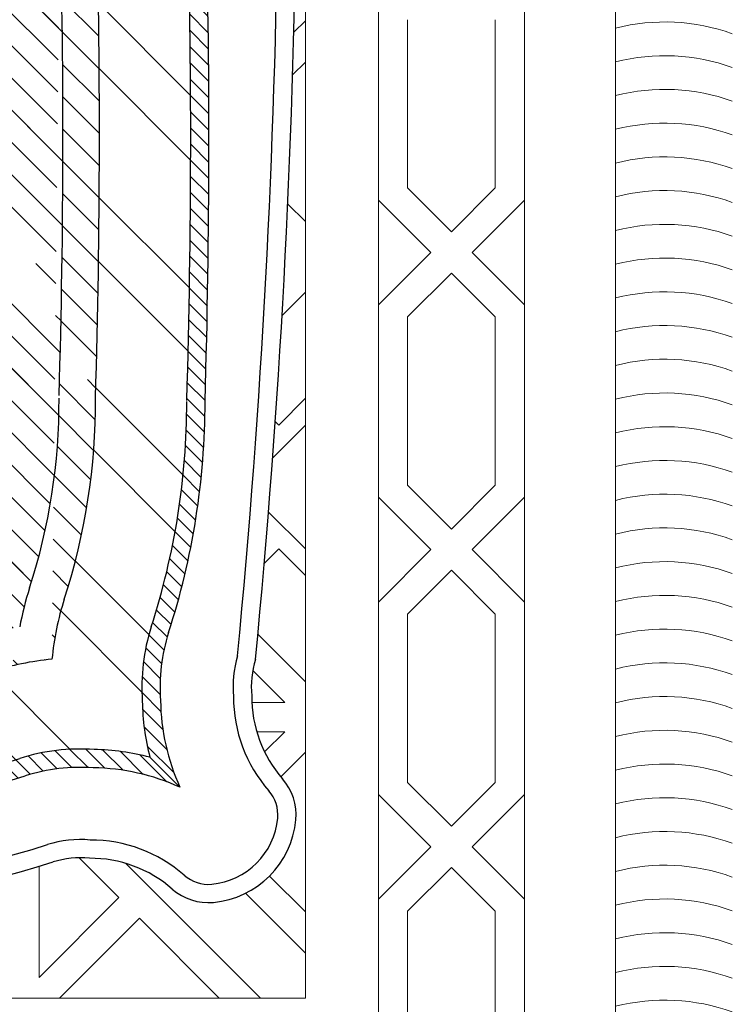
# Model space of a CAD drawing. Units: inches. Extents: x 3592 to 4861, y 1650 to 2243.
# Tile 7 of 30: x 4207.34 to 4219.05, y 1916.11 to 1932.29. Entities that reach past the tile are written whole.
import ezdxf

# ---------------------------------------------------------------- set-up
doc = ezdxf.new("R2010")
doc.units = ezdxf.units.IN
doc.layers.add('A-FURN', color=9, linetype='Continuous', lineweight=13)
doc.layers.add('RA-AP-01$0$INT', color=35, linetype='Continuous', lineweight=5)
for name, color, linetype in [('RA-AP-01$0$FURN', 3, 'Continuous'), ('RA-AP-01$0$WOOD', 64, 'Continuous'), ('RA-AP-02$0$FLPT', 30, 'Continuous')]:
    doc.layers.add(name, color=color, linetype=linetype)

# ---------------------------------------------------------------- blocks, each defined once
blk = doc.blocks.new('A$C67D63ADA')
at = {"layer": 'RA-AP-01$0$INT'}
for p, q in [((5.040068427138238, -6.243416270339336), (5.068754718634292, -6.272102561844619)), ((5.097441010123072, -6.243416270339336), (5.068754718627016, -6.272102561844619)), ((5.202896854247523, -6.243416270324172), (5.231583145752804, -6.272102561820228)), ((5.260269437248857, -6.243416270339973), (5.231583145752802, -6.272102561845255)), ((5.36572528136967, -6.243416270319609), (5.394411572874951, -6.272102561815665)), ((5.394411572874951, -6.272102561815665), (5.423097864372064, -6.243416270309323)), ((5.033441010139864, -6.25941627034044), (4.941240000013775, -6.259416270325027)), ((5.033441010139864, -6.25941627034044), (5.057441010133491, -6.283416270341786)), ((5.104068427125523, -6.259416270336362), (5.080068427127819, -6.283416270341786)), ((5.104068427125523, -6.259416270336362), (5.196269437247836, -6.259416270320948)), ((5.196269437247836, -6.259416270320948), (5.220269437255637, -6.283416270321034)), ((5.266896854244392, -6.259416270343913), (5.242896854253604, -6.283416270342422)), ((5.266896854244392, -6.259416270343913), (5.359097864382099, -6.2594162703285)), ((5.359097864382099, -6.2594162703285), (5.383097864377784, -6.283416270316472)), ((5.405725281375753, -6.283416270312828), (5.429725281365354, -6.259416270315509)), ((5.429725281365354, -6.259416270315509), (5.521926291510647, -6.259416270315509)), ((5.033441010127117, -6.307416270340442), (5.057441010133491, -6.283416270341786)), ((5.104068427130107, -6.307416270336361), (5.080068427127819, -6.283416270341786)), ((5.196269437263445, -6.307416270320947), (5.220269437255637, -6.283416270321034)), ((5.266896854262809, -6.307416270343915), (5.242896854253604, -6.283416270342422)), ((5.359097864373478, -6.307416270328503), (5.383097864377784, -6.283416270316472)), ((5.405725281375753, -6.283416270312828), (5.42972528138643, -6.307416270315791)), ((5.040068427124683, -6.323416270339336), (5.068754718630654, -6.294729978842587)), ((5.097441010136626, -6.323416270339336), (5.068754718630654, -6.294729978842587)), ((5.202896854259693, -6.323416270324171), (5.231583145756439, -6.294729978818199)), ((5.260269437262412, -6.323416270339973), (5.23158314575644, -6.294729978843224)), ((5.36572528138184, -6.323416270319609), (5.394411572878586, -6.294729978813635)), ((5.394411572878586, -6.294729978813635), (5.423097864384927, -6.323416270310751)), ((5.033441010127117, -6.307416270340442), (4.941240000005749, -6.307416270325028)), ((5.104068427130107, -6.307416270336361), (5.196269437263445, -6.307416270320947)), ((5.266896854262809, -6.307416270343915), (5.359097864373478, -6.307416270328503)), ((5.52192629150337, -6.307416270316805), (5.42972528138643, -6.307416270315791)), ((4.877240000006826, -6.363416270330311), (5.477239999992479, -6.363416270332882)), ((4.948123212406629, -6.369730940236769), (4.94180854250045, -6.363416270330588)), ((5.051867417002687, -6.36341627033228), (4.964435959500471, -6.363416270332642)), ((4.964435959500471, -6.363416270332642), (4.971407022735213, -6.370387333567387)), ((5.051867417002686, -6.363416270332284), (5.042215760129571, -6.373067927205397)), ((5.090494834000653, -6.363416270332124), (5.103286866502454, -6.376208302833926)), ((5.148671457508614, -6.363416270331886), (5.090494834000653, -6.363416270332124)), ((5.163298874506619, -6.378043687329889), (5.148671457508651, -6.363416270331923)), ((5.148671457508614, -6.363416270331884), (5.16329887450662, -6.378043687329889)), ((5.181214712156259, -6.381332107981687), (5.163298874506496, -6.363416270331923)), ((5.163298874506496, -6.363416270331923), (5.231181125500023, -6.363416270331545)), ((5.210977238587049, -6.38362015724497), (5.231181125500023, -6.363416270331545)), ((5.245808542497771, -6.363416270331891), (5.231181125499765, -6.378043687329895)), ((5.245808542497771, -6.363416270331893), (5.303985166005732, -6.363416270332143)), ((5.303985166005732, -6.363416270332143), (5.277960454439474, -6.389440981898395)), ((5.3426125830037, -6.363416270332308), (5.356067157592161, -6.376870844920773)), ((5.430044040505915, -6.36341627033268), (5.410388987152561, -6.383071323686029)), ((5.419840115140252, -6.396247612696742), (5.452671457504211, -6.363416270332777)), ((5.477240000007288, -6.923416270324413), (5.477239999992479, -6.363416270332882)), ((5.315298874504621, -6.374729978831223), (5.29779276234004, -6.392236090995803)), ((5.315298874504543, -6.392722141305431), (5.315298874504621, -6.374729978831223)), ((5.331298874504554, -6.390075763711749), (5.33129887450462, -6.374729978831202)), ((5.33129887450462, -6.374729978831202), (5.34234850060876, -6.385779604935344)), ((5.16143007103952, -6.379912490796987), (5.163298874506619, -6.378043687329889)), ((5.239087008324712, -6.385949570154841), (5.231181125499767, -6.378043687329895)), ((5.403480564847417, -6.461744247979447), (5.477239999993128, -6.387984812833736)), ((5.477239999993726, -6.410612229819946), (5.433524271243773, -6.454327958571846)), ((5.477239999996036, -6.498043687322161), (5.433524271243773, -6.454327958571846)), ((5.422210562745039, -6.465641667071083), (5.400410884737611, -6.487441345079475)), ((5.465926291497392, -6.509357395821494), (5.42221056274504, -6.465641667071082)), ((5.405096589283714, -6.509357395823103), (5.465926291497392, -6.509357395821494))]:
    blk.add_line(p, q, dxfattribs=at)
for points in [[(4.877240000006826, -6.19341627032537), (5.647240000006826, -6.19341627032537), (5.647240000006826, -7.09341627032537), (4.877240000006826, -7.09341627032537)], [(4.877240000006826, -6.243416270325369), (5.597240000006826, -6.243416270325369)], [(4.877240000006826, -6.32341627032537), (5.517240000006826, -6.32341627032537), (5.517240000006826, -6.963416270325371), (4.877240000006826, -6.963416270325371)]]:
    blk.add_lwpolyline(points, dxfattribs=at)
for centre, end in [((5.051601958963728, -6.166456270322764), 194.3025426372013), ((5.070081958960181, -6.166456270322764), 194.3025426372013), ((5.088561958964091, -6.16645627032149), 194.3025426378914), ((5.10704195896309, -6.166456270323673), 194.3025426367086), ((5.12552195896209, -6.166456270323673), 194.3025426367086), ((5.144001958965818, -6.1664562703224), 194.3025426373987), ((5.162481958964817, -6.166456270323309), 194.3025426369059), ((5.18096195896127, -6.166456270323309), 194.3025426369059), ((5.19944195896518, -6.166456270322036), 194.3025426375955), ((5.217921958963997, -6.166456270320581), 194.3025426383842), ((5.236401958960631, -6.166456270322946), 194.3025426371027), ((5.25488195896436, -6.166456270322764), 194.3025426372013), ((5.273361958963359, -6.16645627032149), 194.3025426378914), ((5.291841958964723, -6.166456270320217), 194.302542638581), ((5.310321958963722, -6.1664562703224), 194.3025426373987), ((5.328801958965086, -6.166456270322218), 194.3025426374968), ((5.328801958964235, -6.166456270319853), 194.3025426387784), ((5.347281958963233, -6.166456270322036), 194.3025426375955), ((5.365761958962233, -6.166456270322036), 194.3025426375955), ((5.384241958965962, -6.166456270320763), 194.3025426382856), ((5.402721958964961, -6.166456270321672), 194.3025426377928), ((5.421201958961413, -6.166456270321672), 194.3025426377928), ((5.439681958965324, -6.1664562703204), 194.3025426384824), ((5.458161958964141, -6.166456270318944), 194.3025426392711), ((5.476641958960775, -6.166456270321309), 194.3025426379896), ((5.495121958964504, -6.166456270321127), 194.3025426380882), ((5.513601958963502, -6.166456270319853), 194.3025426387784), ((5.532081958964867, -6.166456270318581), 194.3025426394679), ((5.550561958963865, -6.166456270320763), 194.3025426382856), ((5.56904195896523, -6.166456270320581), 194.3025426383842), ((5.587521958961682, -6.166456270318216), 194.3025426396653)]:
    blk.add_arc(centre, 0.1091312342836184, 160.2038431294313, end, dxfattribs=at)
blk = doc.blocks.new('A$C09A87C41')
at = {"layer": 'RA-AP-01$0$WOOD'}
h = blk.add_hatch(dxfattribs=at)
h.set_pattern_fill('ANSI31', color=256, scale=0.05, style=0)
h.set_pattern_definition([(45, (0.7182879904584168, -11.54818755465011), (0.0044194173824159, -0.0044194173824159), [])])
edge = h.paths.add_edge_path()
edge.add_ellipse((5.006516613079209, -11.27459283286495), major_axis=(3.435359877543153, 3.435359877543153), ratio=0.9999999999999982, start_angle=403.3022422558093, end_angle=406.5486575131389, ccw=False)
edge.add_ellipse((5.150455045735207, -6.828790194879051), major_axis=(-0.2901946312779826, 0.2901946312779826), ratio=0.9999999999999875, start_angle=297.2093186994243, end_angle=314.9999999999731, ccw=False)
edge.add_ellipse((5.307117976013378, -6.343033378039902), major_axis=(-0.0707106781186454, 0.0707106781186455), ratio=0.9999999999999651, start_angle=116.7779839927149, end_angle=139.0873288843009)
edge.add_ellipse((5.312718414970339, -6.324818905441738), major_axis=(0.0834173982641243, 0.0834173982641243), ratio=0.9999999999999847, start_angle=225.741775187377, end_angle=249.5633269497028)
edge.add_line((5.361758401537698, -6.432112914518591), (5.345299417747169, -6.448571898309089))
edge.add_ellipse((5.312718414970311, -6.32481890544173), major_axis=(-0.0904884660759946, 0.0904884660759945), ratio=0.9999999999999644, start_angle=135.8720682536374, end_angle=149.7498089726665, ccw=False)
edge.add_ellipse((5.307117976013483, -6.343033378039922), major_axis=(-0.0777817459304867, 0.0777817459304867), ratio=0.9999999999999941, start_angle=117.45144083316339, end_angle=138.9346900893823, ccw=False)
edge.add_ellipse((5.150455045735208, -6.82879019487905), major_axis=(0.2831235634661059, 0.2831235634661059), ratio=0.9999999999999859, start_angle=27.03507540014952, end_angle=44.9867285887044)
edge.add_ellipse((5.006516315412802, -11.27459997798134), major_axis=(-3.428298916554014, 3.428298916554014), ratio=0.9999999999999971, start_angle=-46.70235550375367, end_angle=-43.44815559494434)
edge.add_ellipse((4.743915471599394, -11.2745999779814), major_axis=(3.428298916553931, 3.42829891655393), ratio=0.9999999999999994, start_angle=43.44815559494427, end_angle=46.70235550375375)
edge.add_ellipse((4.599976741276995, -6.828790194879051), major_axis=(0.2831235634661173, 0.2831235634661172), ratio=0.9999999999999861, start_angle=45.01327141129749, end_angle=62.96492459984043)
edge.add_ellipse((4.443313810998718, -6.343033378039922), major_axis=(0.0777817459304893, 0.0777817459304893), ratio=0.9999999999999873, start_angle=221.0653099106178, end_angle=242.54855916687399, ccw=False)
edge.add_ellipse((4.437713372041892, -6.32481890544173), major_axis=(0.0904884660759951, 0.0904884660759951), ratio=0.9999999999999603, start_angle=210.2501910273332, end_angle=224.1279317463614, ccw=False)
edge.add_line((4.405132369265034, -6.448571898309089), (4.388673385474508, -6.432112914518594))
edge.add_ellipse((4.43771337204186, -6.324818905441737), major_axis=(0.0834173982641232, 0.0834173982641232), ratio=0.9999999999999797, start_angle=200.4366730503009, end_angle=224.2582248126243)
edge.add_ellipse((4.443313810998827, -6.343033378039902), major_axis=(-0.0707106781186382, 0.0707106781186382), ratio=0.9999999999999952, start_angle=130.9126711156974, end_angle=153.2220160072772)
edge.add_ellipse((4.599976741276995, -6.828790194879051), major_axis=(-0.2901946312779718, 0.2901946312779718), ratio=0.9999999999999895, start_angle=315.0000000000233, end_angle=332.7906813005773, ccw=False)
edge.add_ellipse((4.743915173933024, -11.27459283286497), major_axis=(-3.435359877543123, 3.435359877543123), ratio=0.9999999999999991, start_angle=313.451342486861, end_angle=316.69775774419077, ccw=False)
edge = h.paths.add_edge_path()
edge.add_ellipse((4.299593848995801, -6.48675334004306), major_axis=(-0.0707106781186556, 0.0707106781186556), ratio=0.9999999999999859, start_angle=206.7779839906583, end_angle=229.0873288838364)
edge.add_ellipse((4.281379376397651, -6.481152901086075), major_axis=(-0.0834173982641623, 0.0834173982641623), ratio=0.9999999999999754, start_angle=225.7417751869729, end_angle=249.5633269497573)
edge.add_line((4.388673385474506, -6.432112914518592), (4.405132369265034, -6.448571898309089))
edge.add_ellipse((4.281379376397657, -6.481152901086004), major_axis=(-0.0904884660760182, 0.0904884660760182), ratio=0.9999999999999957, start_angle=225.8720682533453, end_angle=239.7498089726896, ccw=False)
edge.add_ellipse((4.299593848995796, -6.486753340043026), major_axis=(0.0777817459305317, 0.0777817459305317), ratio=0.9999999999999891, start_angle=297.4514408381613, end_angle=318.9346900891407, ccw=False)
edge.add_ellipse((4.785350665835052, -6.643416270320893), major_axis=(0.2831235634661102, 0.2831235634661102), ratio=0.9999999999999978, start_angle=117.0350753988375, end_angle=152.9649246009711)
edge.add_ellipse((4.299593848995777, -6.800079200598784), major_axis=(-0.0777817459305426, 0.0777817459305426), ratio=0.9999999999999973, start_angle=221.0653099111909, end_angle=242.5485591625442, ccw=False)
edge.add_ellipse((4.281379376397679, -6.805679639555494), major_axis=(-0.0904884660760244, 0.0904884660760244), ratio=0.9999999999999076, start_angle=210.2501910270576, end_angle=224.1279317467988, ccw=False)
edge.add_line((4.405132369264926, -6.838260642332959), (4.388673385474263, -6.854719626123697))
edge.add_ellipse((4.281379376397679, -6.80567963955562), major_axis=(0.0834173982641642, 0.0834173982641642), ratio=0.9999999999999609, start_angle=290.4366730499258, end_angle=314.2582248131156)
edge.add_ellipse((4.299593848995804, -6.800079200598786), major_axis=(-0.0707106781186612, 0.0707106781186612), ratio=0.999999999999977, start_angle=220.9126711163551, end_angle=243.222016008517)
edge.add_ellipse((4.785350665835053, -6.643416270320894), major_axis=(0.2901946312779783, 0.2901946312779783), ratio=0.9999999999999984, start_angle=117.2093186999746, end_angle=152.7906813002342, ccw=False)
edge = h.paths.add_edge_path()
edge.add_ellipse((4.743915471599392, -2.012232562660299), major_axis=(3.428298916553894, 3.428298916553894), ratio=0.9999999999999992, start_angle=223.2976444962459, end_angle=226.5518444050561)
edge.add_ellipse((5.006516315412771, -2.012232562660296), major_axis=(3.428298916553752, 3.428298916553752), ratio=0.9999999999999971, start_angle=223.448155594945, end_angle=226.7023555037531)
edge.add_ellipse((5.150455045735209, -6.458042345762599), major_axis=(0.283123563466111, 0.283123563466111), ratio=0.999999999999996, start_angle=225.0132714112834, end_angle=242.9649246011241)
edge.add_ellipse((5.30711797601273, -6.94379916260194), major_axis=(0.0777817459305174, 0.0777817459305174), ratio=0.9999999999999873, start_angle=401.06530991071423, end_angle=422.548559161793, ccw=False)
edge.add_ellipse((5.312718414969516, -6.962013635200094), major_axis=(0.0904884660760023, 0.0904884660760023), ratio=0.9999999999999566, start_angle=390.2501910269164, end_angle=404.12793174642553, ccw=False)
edge.add_line((5.345299417747278, -6.838260642332959), (5.361758401537942, -6.854719626123698))
edge.add_ellipse((5.312718414969516, -6.962013635200098), major_axis=(0.0834173982641439, 0.0834173982641439), ratio=0.9999999999999785, start_angle=20.43667304973462, end_angle=44.25822481258737)
edge.add_ellipse((5.307117976012772, -6.943799162601948), major_axis=(-0.0707106781186618, 0.0707106781186618), ratio=0.999999999999977, start_angle=-49.08732888421749, end_angle=-26.77798399064677)
edge.add_ellipse((5.150455045735209, -6.458042345762597), major_axis=(0.2901946312779783, 0.2901946312779783), ratio=0.9999999999999957, start_angle=225.0000000000273, end_angle=242.7906812999824, ccw=False)
edge.add_ellipse((5.006516613079198, -2.012239707776725), major_axis=(3.43535987754352, 3.43535987754352), ratio=0.999999999999996, start_angle=223.4513424868609, end_angle=226.697757744191, ccw=False)
edge.add_ellipse((4.743915173933023, -2.012239707776712), major_axis=(3.435359877543229, 3.435359877543229), ratio=0.9999999999999998, start_angle=223.3022422558095, end_angle=226.5486575131387, ccw=False)
edge.add_ellipse((4.599976741276995, -6.458042345762597), major_axis=(0.2901946312779746, 0.2901946312779748), ratio=0.9999999999999964, start_angle=207.2093187000184, end_angle=224.9999999999795, ccw=False)
edge.add_ellipse((4.443313810999427, -6.943799162601947), major_axis=(-0.070710678118668, 0.070710678118668), ratio=0.9999999999999838, start_angle=-63.22201600935903, end_angle=-40.9126711157662)
edge.add_ellipse((4.437713372042683, -6.962013635200099), major_axis=(0.0834173982641484, 0.0834173982641484), ratio=0.9999999999999729, start_angle=45.74177518742643, end_angle=69.56332695026246)
edge.add_line((4.388673385474263, -6.854719626123697), (4.405132369264926, -6.838260642332958))
edge.add_ellipse((4.437713372042681, -6.962013635200094), major_axis=(0.0904884660760224, 0.0904884660760225), ratio=0.9999999999999282, start_angle=405.87206825357924, end_angle=419.7498089730807, ccw=False)
edge.add_ellipse((4.443313810999475, -6.94379916260194), major_axis=(-0.0777817459305165, 0.0777817459305165), ratio=0.9999999999999927, start_angle=297.4514408382556, end_angle=318.93469008929503, ccw=False)
edge.add_ellipse((4.599976741276995, -6.458042345762597), major_axis=(0.2831235634661077, 0.2831235634661077), ratio=0.9999999999999937, start_angle=207.0350753988627, end_angle=224.9867285886981)
edge = h.paths.add_edge_path()
edge.add_ellipse((5.450837938016399, -6.800079200598789), major_axis=(-0.0707106781186565, 0.0707106781186565), ratio=0.9999999999999875, start_angle=26.77798399147072, end_angle=49.08732888364846)
edge.add_ellipse((5.469052410614524, -6.80567963955562), major_axis=(0.0834173982641601, 0.0834173982641601), ratio=0.9999999999999984, start_angle=135.7417751868887, end_angle=159.563326950074)
edge.add_line((5.36175840153794, -6.854719626123697), (5.345299417747278, -6.838260642332959))
edge.add_ellipse((5.469052410614523, -6.805679639555488), major_axis=(0.0904884660760307, 0.0904884660760307), ratio=0.9999999999999984, start_angle=135.8720682531977, end_angle=149.7498089729454, ccw=False)
edge.add_ellipse((5.450837938016426, -6.800079200598787), major_axis=(0.0777817459305426, 0.0777817459305427), ratio=0.9999999999999968, start_angle=117.4514408374904, end_angle=138.9346900888003, ccw=False)
edge.add_ellipse((4.965081121177151, -6.643416270320895), major_axis=(-0.2831235634661119, 0.2831235634661119), ratio=0.9999999999999992, start_angle=207.0350753990193, end_angle=242.9649246011595)
edge.add_ellipse((5.450837938016407, -6.486753340043026), major_axis=(0.0777817459305285, 0.0777817459305285), ratio=0.9999999999999747, start_angle=131.0653099108597, end_angle=152.5485591618505, ccw=False)
edge.add_ellipse((5.469052410614547, -6.481152901086004), major_axis=(0.09048846607603, 0.09048846607603), ratio=0.9999999999999619, start_angle=120.25019102731059, end_angle=134.1279317466551, ccw=False)
edge.add_line((5.345299417747169, -6.448571898309089), (5.361758401537697, -6.432112914518592))
edge.add_ellipse((5.469052410614551, -6.481152901086075), major_axis=(-0.0834173982641603, 0.0834173982641603), ratio=0.9999999999999998, start_angle=20.43667305024269, end_angle=44.25822481302925)
edge.add_ellipse((5.450837938016403, -6.486753340043062), major_axis=(-0.0707106781186603, 0.0707106781186603), ratio=0.9999999999999737, start_angle=40.91267111616517, end_angle=63.22201600943157)
edge.add_ellipse((4.965081121177149, -6.643416270320895), major_axis=(0.2901946312779771, 0.2901946312779771), ratio=0.9999999999999992, start_angle=297.2093186997686, end_angle=332.7906813000034, ccw=False)
h = blk.add_hatch(dxfattribs=at)
h.set_pattern_fill('ANSI32', color=256, scale=0.2, style=0)
h.set_pattern_definition([(45, (0.7182879904584168, -11.54818755465011), (0.0530330085889911, -0.0530330085889911), []), (45, (0.7182879904584168, -11.51283221565011), (0.0530330085889911, -0.0530330085889911), [])])
edge = h.paths.add_edge_path()
edge.add_ellipse((5.15045504573521, -6.82879019487905), major_axis=(-0.2831235634661157, 0.2831235634661156), ratio=0.9999999999999889, start_angle=297.21454354460053, end_angle=314.98672858870884, ccw=False)
edge.add_ellipse((5.307117976013485, -6.343033378039922), major_axis=(-0.0777817459304881, 0.0777817459304881), ratio=0.9999999999999928, start_angle=116.7981781115797, end_angle=138.9346900893818)
edge.add_ellipse((5.312718414970311, -6.32481890544173), major_axis=(-0.0904884660759946, 0.0904884660759946), ratio=0.9999999999999658, start_angle=135.8720682536378, end_angle=149.7498089726664)
edge.add_ellipse((5.469052410614547, -6.481152901086004), major_axis=(0.0904884660760303, 0.0904884660760302), ratio=0.9999999999999603, start_angle=120.2501910273106, end_angle=134.1279317466551)
edge.add_ellipse((5.450837938016407, -6.486753340043026), major_axis=(-0.0777817459305327, 0.0777817459305327), ratio=0.9999999999999915, start_angle=41.06530991085969, end_angle=63.20182189333976)
edge.add_ellipse((4.965081121177151, -6.643416270320894), major_axis=(-0.2831235634661133, 0.2831235634661133), ratio=0.9999999999999984, start_angle=207.214543545815, end_angle=242.7854564539869, ccw=False)
edge.add_ellipse((5.450837938016426, -6.800079200598786), major_axis=(0.0777817459305424, 0.0777817459305424), ratio=0.9999999999999962, start_angle=116.7981781073729, end_angle=138.9346900888086)
edge.add_ellipse((5.469052410614524, -6.805679639555493), major_axis=(0.0904884660760289, 0.0904884660760289), ratio=0.9999999999999841, start_angle=135.872068253202, end_angle=149.7498089729424)
edge.add_ellipse((5.312718414969522, -6.962013635200094), major_axis=(-0.0904884660760224, 0.0904884660760225), ratio=0.9999999999999282, start_angle=-59.7498089730807, end_angle=-45.87206825357926)
edge.add_ellipse((5.307117976012728, -6.94379916260194), major_axis=(0.0777817459305181, 0.0777817459305181), ratio=0.9999999999999861, start_angle=41.06530991070497, end_angle=63.20182189334603)
edge.add_ellipse((5.150455045735208, -6.458042345762599), major_axis=(0.2831235634661146, 0.2831235634661146), ratio=0.9999999999999907, start_angle=225.013271411291, end_angle=242.7854564539341, ccw=False)
edge.add_ellipse((5.006516315412806, -2.012232562660296), major_axis=(3.428298916554143, 3.428298916554143), ratio=0.9999999999999941, start_angle=223.4481555949448, end_angle=226.7023555037533, ccw=False)
edge.add_ellipse((4.743915471599424, -2.012232562660299), major_axis=(3.428298916554168, 3.428298916554171), ratio=0.9999999999999991, start_angle=223.2976444962462, end_angle=226.551844405056, ccw=False)
edge.add_ellipse((4.599976741276996, -6.458042345762597), major_axis=(0.2831235634661098, 0.2831235634661098), ratio=0.9999999999999973, start_angle=207.2145435460398, end_angle=224.9867285887048, ccw=False)
edge.add_ellipse((4.443313810999473, -6.94379916260194), major_axis=(-0.0777817459305183, 0.0777817459305183), ratio=0.9999999999999823, start_angle=-63.2018218932521, end_angle=-41.06530991071377)
edge.add_ellipse((4.437713372042686, -6.962013635200094), major_axis=(-0.0904884660760028, 0.0904884660760028), ratio=0.9999999999999504, start_angle=-44.12793174642511, end_angle=-30.25019102691602)
edge.add_ellipse((4.281379376397679, -6.80567963955549), major_axis=(-0.0904884660760215, 0.0904884660760215), ratio=0.9999999999999245, start_angle=210.2501910270558, end_angle=224.1279317467963)
edge.add_ellipse((4.299593848995777, -6.800079200598786), major_axis=(0.077781745930539, 0.077781745930539), ratio=0.999999999999963, start_angle=311.0653099111909, end_angle=333.2018218926339)
edge.add_ellipse((4.785350665835052, -6.643416270320894), major_axis=(0.2831235634661089, 0.2831235634661091), ratio=0.9999999999999989, start_angle=117.21454354600829, end_angle=152.7854564541833, ccw=False)
edge.add_ellipse((4.299593848995796, -6.486753340043026), major_axis=(0.077781745930533, 0.077781745930533), ratio=0.9999999999999792, start_angle=296.7981781066777, end_angle=318.9346900891398)
edge.add_ellipse((4.281379376397657, -6.481152901086003), major_axis=(-0.0904884660760217, 0.0904884660760217), ratio=0.9999999999999742, start_angle=225.872068253344, end_angle=239.7498089726891)
edge.add_ellipse((4.437713372041892, -6.32481890544173), major_axis=(0.090488466075997, 0.090488466075997), ratio=0.9999999999999756, start_angle=210.2501910273331, end_angle=224.1279317463622)
edge.add_ellipse((4.44331381099872, -6.343033378039923), major_axis=(0.0777817459304873, 0.0777817459304872), ratio=0.9999999999999861, start_angle=221.0653099106177, end_angle=243.2018218883976)
edge.add_ellipse((4.599976741276995, -6.828790194879051), major_axis=(-0.2831235634661067, 0.2831235634661067), ratio=0.9999999999999895, start_angle=315.01327141129775, end_angle=332.78545645540567, ccw=False)
edge.add_ellipse((4.743915471599392, -11.2745999779814), major_axis=(-3.428298916553902, 3.428298916553902), ratio=0.9999999999999984, start_angle=313.4481555949443, end_angle=316.7023555037538, ccw=False)
edge.add_ellipse((5.006516315412786, -11.27459997798134), major_axis=(-3.428298916554052, 3.428298916554052), ratio=1, start_angle=313.29764449624645, end_angle=316.5518444050555, ccw=False)
edge = h.paths.add_edge_path(flags=16)
edge.add_ellipse((4.745320840887742, -11.27459782170807), major_axis=(3.392940520945516, 3.392940520945516), ratio=1, start_angle=43.44876692339471, end_angle=46.71249975461917)
edge.add_ellipse((4.599976741276995, -6.828790194878992), major_axis=(-0.2477682244067734, 0.2477682244067734), ratio=0.9999999999999911, start_angle=-45.31868720933983, end_angle=-27.00912183057358)
edge.add_ellipse((4.443313810998828, -6.343033378039872), major_axis=(0.1131370849898469, 0.1131370849898469), ratio=0.9999999999999724, start_angle=230.5682590208478, end_angle=242.6218359751805, ccw=False)
edge.add_ellipse((4.299593848995757, -6.486753340043112), major_axis=(-0.1131370849898624, 0.1131370849898624), ratio=0.9999999999999953, start_angle=207.3781640250758, end_angle=219.4317409792351, ccw=False)
edge.add_ellipse((4.78535066583505, -6.643416270320884), major_axis=(0.2477682244067863, 0.2477682244067863), ratio=0.9999999999999974, start_angle=117.0091218305267, end_angle=152.9908781690427)
edge.add_ellipse((4.299593848995773, -6.800079200598856), major_axis=(0.1131370849898833, 0.1131370849898833), ratio=0.9999999999999682, start_angle=320.56825902084296, end_angle=332.62183597593753, ccw=False)
edge.add_ellipse((4.443313810999473, -6.943799162601939), major_axis=(0.1131370849898351, 0.1131370849898351), ratio=0.9999999999999213, start_angle=387.3781640246361, end_angle=399.43174097937606, ccw=False)
edge.add_ellipse((4.599976741276996, -6.458042345762606), major_axis=(0.2477682244067743, 0.2477682244067742), ratio=0.99999999999999, start_angle=207.0091218307682, end_angle=225.3186872093523)
edge.add_ellipse((4.745320840887777, -2.012234718933553), major_axis=(-3.392940520945741, 3.392940520945741), ratio=0.9999999999999992, start_angle=133.2875002453813, end_angle=136.5512330766047)
edge.add_ellipse((5.005110946124445, -2.012234718933546), major_axis=(3.392940520945412, 3.392940520945411), ratio=0.9999999999999989, start_angle=223.4487669233947, end_angle=226.7124997546191)
edge.add_ellipse((5.150455045735207, -6.458042345762608), major_axis=(-0.2477682244067739, 0.2477682244067739), ratio=0.9999999999999966, start_angle=134.6813127906568, end_angle=152.9908781692236)
edge.add_ellipse((5.30711797601273, -6.943799162601939), major_axis=(-0.1131370849898406, 0.1131370849898406), ratio=0.9999999999999811, start_angle=320.568259020624, end_angle=332.62183597538194, ccw=False)
edge.add_ellipse((5.45083793801643, -6.800079200598855), major_axis=(0.113137084989895, 0.113137084989895), ratio=0.999999999999955, start_angle=117.3781640240419, end_angle=129.4317409791577, ccw=False)
edge.add_ellipse((4.965081121177152, -6.643416270320884), major_axis=(0.2477682244067847, 0.2477682244067847), ratio=0.9999999999999992, start_angle=297.0091218309669, end_angle=332.990878169475)
edge.add_ellipse((5.450837938016447, -6.486753340043118), major_axis=(-0.1131370849898789, 0.1131370849898789), ratio=0.9999999999999342, start_angle=50.56825902076281, end_angle=62.62183597491821, ccw=False)
edge.add_ellipse((5.30711797601337, -6.34303337803987), major_axis=(0.1131370849898374, 0.1131370849898374), ratio=0.9999999999999493, start_angle=207.3781640247929, end_angle=219.4317409791543, ccw=False)
edge.add_ellipse((5.150455045735204, -6.828790194878992), major_axis=(-0.2477682244067807, 0.2477682244067808), ratio=0.9999999999999934, start_angle=-62.99087816941401, end_angle=-44.68131279065508)
edge.add_ellipse((5.005110946124442, -11.27459782170805), major_axis=(3.392940520945543, 3.392940520945543), ratio=0.9999999999999974, start_angle=43.28750024538099, end_angle=46.55123307660507)
edge = h.paths.add_edge_path(flags=0)
edge.add_ellipse((4.745321446260899, -11.27461227828643), major_axis=(3.378818834290158, 3.378818834290157), ratio=0.9999999999999996, start_angle=43.44228925150885, end_angle=46.72161971502517)
edge.add_ellipse((4.599976741276998, -6.828790194878991), major_axis=(-0.2336260887830454, 0.2336260887830454), ratio=0.9999999999999974, start_angle=-45.30974264369766, end_angle=-26.99844483641433)
edge.add_ellipse((4.443313810998811, -6.343033378039858), major_axis=(0.1272792206135962, 0.1272792206135962), ratio=0.9999999999999403, start_angle=235.6264990356023, end_angle=242.6432427499436, ccw=False)
edge.add_ellipse((4.299593848995773, -6.486753340043007), major_axis=(0.1272792206136285, 0.1272792206136286), ratio=0.9999999999999204, start_angle=297.35675724967757, end_angle=304.3735009644582, ccw=False)
edge.add_ellipse((4.785350665835048, -6.643416270320905), major_axis=(0.2336260887830504, 0.2336260887830504), ratio=0.9999999999999921, start_angle=116.998444836676, end_angle=153.0015551636886)
edge.add_ellipse((4.299593848995741, -6.800079200598703), major_axis=(-0.1272792206136906, 0.1272792206136906), ratio=0.9999999999996289, start_angle=235.62649903554922, end_angle=242.64324274961962, ccw=False)
edge.add_ellipse((4.443313810999469, -6.943799162601998), major_axis=(-0.1272792206136219, 0.1272792206136219), ratio=0.9999999999999658, start_angle=297.3567572500489, end_angle=304.3735009646209, ccw=False)
edge.add_ellipse((4.599976741276995, -6.458042345762605), major_axis=(0.2336260887830445, 0.2336260887830445), ratio=0.9999999999999957, start_angle=206.9984448365414, end_angle=225.3097426436968)
edge.add_ellipse((4.745321446260921, -2.012220262355212), major_axis=(3.378818834290089, 3.378818834290088), ratio=0.9999999999999994, start_angle=223.2783802849744, end_angle=226.5577107484907)
edge.add_ellipse((5.005110340751275, -2.012220262355198), major_axis=(3.378818834290274, 3.378818834290274), ratio=0.9999999999999992, start_angle=223.4422892515091, end_angle=226.7216197150253)
edge.add_ellipse((5.150455045735206, -6.458042345762609), major_axis=(0.2336260887830463, 0.2336260887830463), ratio=0.9999999999999937, start_angle=224.6902573562994, end_angle=243.0015551634542)
edge.add_ellipse((5.30711797601273, -6.943799162602), major_axis=(-0.1272792206135949, 0.1272792206135949), ratio=0.9999999999997138, start_angle=325.62649903537766, end_angle=332.6432427499585, ccw=False)
edge.add_ellipse((5.450837938016461, -6.800079200598699), major_axis=(-0.1272792206135936, 0.1272792206135936), ratio=0.999999999999666, start_angle=27.356757250387716, end_angle=34.37350096445232, ccw=False)
edge.add_ellipse((4.965081121177155, -6.643416270320904), major_axis=(0.23362608878305, 0.23362608878305), ratio=0.9999999999999992, start_angle=296.9984448363078, end_angle=333.0015551633219)
edge.add_ellipse((5.450837938016428, -6.486753340043003), major_axis=(0.1272792206136045, 0.1272792206136045), ratio=0.9999999999999529, start_angle=145.6264990355431, end_angle=152.6432427503271, ccw=False)
edge.add_ellipse((5.307117976013396, -6.34303337803986), major_axis=(0.1272792206135615, 0.1272792206135615), ratio=0.9999999999996925, start_angle=207.3567572500474, end_angle=214.3735009643965, ccw=False)
edge.add_ellipse((5.150455045735208, -6.828790194878991), major_axis=(-0.2336260887830484, 0.2336260887830485), ratio=0.9999999999999953, start_angle=-63.00155516358085, end_angle=-44.69025735630093)
edge.add_ellipse((5.005110340751286, -11.27461227828636), major_axis=(-3.378818834290266, 3.378818834290266), ratio=0.9999999999999998, start_angle=-46.72161971502535, end_angle=-43.44228925150914)
edge = h.paths.add_edge_path(flags=0)
edge.add_ellipse((4.747128261062206, -11.27459926241731), major_axis=(-3.343445075648777, 3.343445075648777), ratio=0.9999999999999991, start_angle=-46.55229325491085, end_angle=-43.26504392007965)
edge.add_ellipse((4.599976741277094, -6.828790194878977), major_axis=(0.198270749723715, 0.198270749723715), ratio=0.999999999999988, start_angle=44.18347671010175, end_angle=62.12936993332099)
edge.add_ellipse((4.785350665835048, -6.643416270320889), major_axis=(0.198270749723727, 0.198270749723727), ratio=0.9999999999999971, start_angle=117.8706300667295, end_angle=152.1293699332338)
edge.add_ellipse((4.599976741276998, -6.458042345762598), major_axis=(0.1982707497237202, 0.1982707497237202), ratio=0.9999999999999882, start_angle=207.8706300666892, end_angle=225.8165232899116)
edge.add_ellipse((4.747128261062279, -2.01223327822427), major_axis=(-3.343445075648579, 3.34344507564858), ratio=0.9999999999999984, start_angle=133.2650439200784, end_angle=136.5522932549098)
edge.add_ellipse((5.003303525949927, -2.012233278224277), major_axis=(-3.343445075648679, 3.343445075648679), ratio=0.9999999999999996, start_angle=133.4477067450899, end_angle=136.7349560799216)
edge.add_ellipse((5.150455045735204, -6.458042345762598), major_axis=(-0.1982707497237223, 0.1982707497237223), ratio=0.9999999999999994, start_angle=134.1834767100914, end_angle=152.1293699333112)
edge.add_ellipse((4.965081121177155, -6.643416270320892), major_axis=(0.1982707497237268, 0.1982707497237267), ratio=0.9999999999999987, start_angle=297.8706300667671, end_angle=332.1293699332712)
edge.add_ellipse((5.150455045735109, -6.828790194878977), major_axis=(0.1982707497237106, 0.1982707497237105), ratio=0.9999999999999982, start_angle=27.87063006667902, end_angle=45.8165232898948)
edge.add_ellipse((5.00330352595001, -11.2745992624173), major_axis=(3.343445075648743, 3.343445075648743), ratio=0.9999999999999996, start_angle=43.26504392007961, end_angle=46.55229325491089)
edge = h.paths.add_edge_path(flags=0)
edge.add_ellipse((4.747685770081003, -11.27459857725902), major_axis=(3.329301968186143, 3.329301968186141), ratio=0.9999999999999989, start_angle=43.44789769190167, end_angle=46.74269456932172)
edge.add_ellipse((4.599976741277087, -6.828790194878972), major_axis=(-0.1841286140999701, 0.1841286140999702), ratio=0.9999999999999841, start_angle=-45.99531238101485, end_angle=-30.22398030679106)
edge.add_ellipse((4.785350665835029, -6.643416270320906), major_axis=(0.1841286140999794, 0.1841286140999793), ratio=0.9999999999999998, start_angle=120.2239803068321, end_angle=149.7760196931203)
edge.add_ellipse((4.599976741276998, -6.458042345762589), major_axis=(0.1841286140999956, 0.1841286140999956), ratio=0.9999999999999953, start_angle=210.2239803068005, end_angle=225.9953123810239)
edge.add_ellipse((4.747685770081015, -2.012233963382593), major_axis=(-3.329301968186209, 3.32930196818621), ratio=0.9999999999999991, start_angle=133.2573054306775, end_angle=136.5521023080975)
edge.add_ellipse((5.002746016931159, -2.012233963382618), major_axis=(-3.329301968186245, 3.329301968186245), ratio=0.9999999999999984, start_angle=133.447897691902, end_angle=136.7426945693227)
edge.add_ellipse((5.150455045735208, -6.458042345762592), major_axis=(-0.1841286140999912, 0.1841286140999912), ratio=0.9999999999999873, start_angle=134.0046876189747, end_angle=149.7760196931988)
edge.add_ellipse((4.965081121177172, -6.643416270320907), major_axis=(-0.1841286140999788, 0.1841286140999788), ratio=0.9999999999999968, start_angle=210.2239803068796, end_angle=239.7760196931682)
edge.add_ellipse((5.150455045735117, -6.82879019487897), major_axis=(0.1841286140999714, 0.1841286140999713), ratio=0.9999999999999896, start_angle=30.22398030679139, end_angle=45.99531238102014)
edge.add_ellipse((5.002746016931209, -11.274598577259), major_axis=(3.329301968186158, 3.329301968186158), ratio=1, start_angle=43.25730543067866, end_angle=46.5521023080979)
h = blk.add_hatch(dxfattribs=at)
h.set_pattern_fill('ANSI31', color=256, scale=0.1, style=0)
h.set_pattern_definition([(45, (0.7182879904584168, -11.54818755465011), (0.0088388347648318, -0.0088388347648318), [])])
edge = h.paths.add_edge_path(flags=16)
edge.add_arc((4.965081121177173, -6.643416270320907), 0.2603971832811541, 345.2239803068796, 374.7760196931681)
edge.add_arc((4.965081121177173, -6.643416270320907), 0.2603971832811541, -14.776019693120418, 14.77601969316811, ccw=False)
edge = h.paths.add_edge_path(flags=16)
edge.add_arc((4.785350665835029, -6.643416270320907), 0.2603971832811541, 165.223980306832, 194.7760196931204)
edge.add_arc((4.785350665835029, -6.643416270320907), 0.2603971832811541, 165.223980306832, 194.7760196931204, ccw=False)
edge = h.paths.add_edge_path(flags=0)
edge.add_arc((4.785350665835029, -6.643416270320907), 0.2603971832811541, 165.223980306832, 194.7760196931204)
edge.add_arc((4.785350665835029, -6.643416270320907), 0.2603971832811541, 165.223980306832, 194.7760196931204, ccw=False)
edge = h.paths.add_edge_path(flags=0)
edge.add_arc((4.785350665835029, -6.643416270320907), 0.2603971832811541, 165.223980306832, 194.7760196931204)
edge.add_arc((4.785350665835029, -6.643416270320907), 0.2603971832811541, 165.223980306832, 194.7760196931204, ccw=False)
edge = h.paths.add_edge_path(flags=0)
edge.add_arc((4.785350665835029, -6.643416270320907), 0.2603971832811541, 165.223980306832, 194.7760196931204)
edge.add_arc((4.785350665835029, -6.643416270320907), 0.2603971832811541, 165.223980306832, 194.7760196931204, ccw=False)
edge = h.paths.add_edge_path(flags=0)
edge.add_arc((4.785350665835029, -6.643416270320907), 0.2603971832811541, 165.223980306832, 194.7760196931204)
edge.add_arc((4.785350665835029, -6.643416270320907), 0.2603971832811541, 165.223980306832, 194.7760196931204, ccw=False)
edge = h.paths.add_edge_path(flags=0)
edge.add_arc((4.785350665835029, -6.643416270320907), 0.2603971832811541, 165.223980306832, 194.7760196931204)
edge.add_arc((4.785350665835029, -6.643416270320907), 0.2603971832811541, 165.223980306832, 194.7760196931204, ccw=False)
edge = h.paths.add_edge_path(flags=0)
edge.add_arc((4.785350665835029, -6.643416270320907), 0.2603971832811541, 165.223980306832, 194.7760196931204)
edge.add_arc((4.785350665835029, -6.643416270320907), 0.2603971832811541, 165.223980306832, 194.7760196931204, ccw=False)
edge = h.paths.add_edge_path()
edge.add_arc((5.30711797601273, -6.943799162601939), 0.1599999999999918, 95.56825902062381, 107.6218359753744)
edge.add_arc((5.150455045735207, -6.458042345762605), 0.3503971832811637, 269.6813127906517, 287.9908781692269)
edge.add_arc((5.307117976013371, -6.34303337803987), 0.1599999999999917, 252.3781640232651, 264.4317409791539)
edge.add_arc((4.965081121177153, -6.643416270320884), 0.3503971832811761, 342.0091218309644, 377.9908781694648)
edge.add_arc((5.005110946124438, -2.012234718933557), 4.798342501046485, 268.4423197280547, 271.7124997546188)
edge.add_arc((5.150455045735207, -6.828790194878991), 0.3503971832811637, 72.00912183077308, 90.31868720934834)
edge.add_arc((5.005110340751293, -2.012220262355208), 4.778371420254705, 268.433225420277, 271.7034061068158)
edge.add_arc((5.150455045735207, -6.828790194878991), 0.3303971832811637, 72.00912183077308, 90.31868720934834)
edge.add_arc((5.005110340751291, -11.27461227828638), 4.7783714202547, 88.29659389318418, 91.5667745797229)
edge.add_arc((5.450837938016446, -6.486753340043115), 0.1600000000000254, 185.5682590207637, 197.6218359749416)
edge.add_arc((5.450837938016429, -6.800079200598855), 0.1600000000000541, 162.3781640240467, 174.4317409791574)
edge.add_arc((5.307117976012735, -6.943799162601998), 0.1800000000000505, 100.6264990353792, 107.6432427499818)
edge.add_arc((5.307117976013394, -6.343033378039859), 0.1800000000000069, 252.3567572486067, 259.3735009643972)
edge.add_arc((5.45083793801643, -6.486753340043007), 0.1800000000000424, 190.6264990355417, 197.6432427503393)
edge.add_arc((4.965081121177155, -6.643416270320905), 0.3303971832811676, 341.9984448362978, 378.0015551633146)
edge.add_arc((5.450837938016462, -6.800079200598699), 0.1800000000000547, 162.3567572504062, 169.373500964452)
edge.add_arc((5.150455045735206, -6.458042345762599), 0.2803971832811691, 269.1834767100981, 287.1293699333106)
edge.add_arc((5.150455045735107, -6.828790194878977), 0.2803971832811534, 72.87063006667864, 90.81652328989695)
edge.add_arc((4.965081121177155, -6.643416270320891), 0.2803971832811769, 342.8706300667665, 377.1293699332709)
edge.add_arc((5.150455045735205, -6.45804234576259), 0.2603971832811776, 269.0046876189688, 284.7760196931993)
edge.add_arc((5.150455045735117, -6.828790194878972), 0.2603971832811458, 75.22398030679119, 90.99531238102313)
edge.add_arc((5.150455045735207, -6.458042345762605), 0.3303971832811637, 269.6813127906517, 287.9908781692269)
edge.add_arc((5.003303525949946, -2.012233278224274), 4.728345371032053, 268.4320043718199, 271.7349560799219)
edge.add_arc((5.003303525949998, -11.27459926241731), 4.728345371032045, 88.2650439200796, 91.56799562818075)
edge.add_arc((5.00274601693117, -2.012233963382607), 4.708343996644348, 268.4295004240392, 271.7426945693223)
edge.add_arc((5.002746016931202, -11.274598577259), 4.708343996644358, 88.25730543067873, 91.57049957596126)
edge.add_arc((4.747685770080999, -11.274598577259), 4.708343996644359, 88.42950042403872, 91.74269456932127)
edge.add_arc((4.747685770081036, -2.012233963382596), 4.708343996644359, 268.2573054306777, 271.5704995759608)
edge.add_arc((4.747128261062202, -11.27459926241732), 4.728345371032054, 88.43200437181925, 91.73495607992041)
edge.add_arc((4.747128261062259, -2.012233278224274), 4.728345371032054, 268.265043920078, 271.56799562818)
edge.add_arc((4.74532144626091, -11.27461227828638), 4.778371420254699, 88.43322542027705, 91.7034061068158)
edge.add_arc((4.599976741276996, -6.828790194878991), 0.3303971832811637, 89.68131279065165, 107.9908781692269)
edge.add_arc((4.599976741276996, -6.458042345762605), 0.3303971832811637, 252.0091218307731, 270.3186872093484)
edge.add_arc((4.745321446260912, -2.012220262355208), 4.778371420254705, 268.2965938931842, 271.5667745797229)
edge.add_arc((4.599976741276996, -6.828790194878991), 0.3503971832811637, 89.68131279065165, 107.9908781692269)
edge.add_arc((4.745320840887767, -2.012234718933562), 4.79834250104648, 268.2875002453812, 271.5576802719454)
edge.add_arc((4.599976741277086, -6.828790194878972), 0.2603971832811458, 89.00468761897682, 104.7760196932087)
edge.add_arc((4.599976741276998, -6.45804234576259), 0.2603971832811776, 255.2239803068007, 270.9953123810312)
edge.add_arc((4.785350665835048, -6.643416270320891), 0.2803971832811769, 162.8706300667291, 197.1293699332334)
edge.add_arc((4.599976741277096, -6.828790194878977), 0.2803971832811534, 89.183476710103, 107.1293699333213)
edge.add_arc((4.599976741276996, -6.458042345762599), 0.2803971832811691, 252.8706300666894, 270.816523289902)
edge.add_arc((4.299593848995741, -6.800079200598699), 0.1800000000000547, 10.626499035548, 17.64324274959381)
edge.add_arc((4.785350665835048, -6.643416270320905), 0.3303971832811676, 161.9984448366853, 198.0015551637021)
edge.add_arc((4.299593848995773, -6.486753340043007), 0.1800000000000424, 342.3567572496606, 349.3735009644582)
edge.add_arc((4.44331381099881, -6.343033378039859), 0.1800000000000069, 280.6264990356027, 287.6432427513933)
edge.add_arc((4.443313810999468, -6.943799162601998), 0.1800000000000505, 72.35675725001818, 79.37350096462075)
edge.add_arc((4.299593848995773, -6.800079200598855), 0.1600000000000541, 5.568259020842612, 17.62183597595322)
edge.add_arc((4.78535066583505, -6.643416270320884), 0.3503971832811761, 162.0091218305351, 197.9908781690354)
edge.add_arc((4.299593848995757, -6.486753340043115), 0.1600000000000254, 342.3781640250583, 354.4317409792362)
edge.add_arc((4.443313810998832, -6.34303337803987), 0.1599999999999917, 275.5682590208461, 287.6218359767349)
edge.add_arc((4.599976741276996, -6.458042345762605), 0.3503971832811637, 252.0091218307731, 270.3186872093484)
edge.add_arc((4.443313810999473, -6.943799162601939), 0.1599999999999918, 72.37816402462555, 84.43174097937616)
edge.add_arc((5.005110946124436, -11.27459782170804), 4.798342501046482, 88.28750024538114, 91.55768027194539)
edge.add_arc((4.745320840887765, -11.27459782170804), 4.798342501046489, 88.44231972805461, 91.7124997546188)
blk.add_line((5.345299417747169, -6.448571898309089), (5.361758401537697, -6.432112914518592), dxfattribs=at)
blk.add_line((5.345299417747169, -6.448571898309089), (5.361758401537697, -6.432112914518592), dxfattribs=at)
for centre, radius, start, end in [((4.822367809588968, -11.24386377427369), 4.875754844654793, 84.47541031816009, 89.38149865164627), ((5.37685568118924, -6.398500391533074), 0.0300000000000001, 84.74312400453641, 131.228949079599), ((5.375023258723073, -6.418416270321089), 0.0499999999998357, 5.256875994505274, 84.74312400476296), ((5.312286627958059, -6.32481890544176), 0.067970015963027, 269.4666929485871, 311.2289490796011), ((4.822367809588968, -11.24386377427369), 4.865754844654794, 84.4870438419231, 89.38149865164627), ((5.376855681189239, -6.398500391533072), 0.0199999999999982, 84.74312400452995, 131.2289490795956), ((5.375023258723052, -6.41841627032111), 0.0399999999998586, 5.256875994532665, 84.74312400479155), ((5.312286627958155, -6.324818905441724), 0.0779700159629894, 269.8623536995577, 311.2289490795309), ((5.306686189001188, -6.34303337803988), 0.0500000000000019, 252.644316024698, 275.7020707653122), ((5.306686189001212, -6.343033378039901), 0.0599999999999777, 253.6788686698736, 275.1761921612389), ((5.006516613079189, -11.27459283286492), 4.858332530454211, 88.302242255809, 91.54738399976372), ((5.150455045735209, -6.828790194879051), 0.4103971832811724, 72.04030024487774, 89.99999999997355), ((5.394939137511138, -6.416583847854957), 0.019999999999953, 318.7710509202994, 5.256875994224816), ((5.39493913751109, -6.416583847854941), 0.0299999999999995, 318.7710509203566, 5.256875994279804), ((5.006516315412803, -11.27459997798136), 4.848346823659694, 88.3067023394723, 91.55184440505565), ((5.150455045735209, -6.828790194879051), 0.4003971832811724, 72.04030024487774, 89.99999999997355), ((5.46862062360236, -6.481152901086179), 0.077970015963032, 138.7710509203579, 180.1376463009859), ((5.312718414970341, -6.324818905441737), 0.117970015963001, 270.741775187375, 294.5633269497008), ((5.469052410614551, -6.481152901086075), 0.1179700159630533, 155.4366730502426, 179.2582248130275), ((5.307117976013377, -6.343033378039901), 0.0999999999999796, 252.4716349535609, 274.0873288843005), ((5.468620623602355, -6.481152901086177), 0.0679700159630267, 138.7710509203559, 180.5333070513694), ((5.307117976013483, -6.343033378039922), 0.1099999999999514, 252.4514408345641, 273.9346900893823), ((5.312718414970311, -6.32481890544173), 0.127970015963015, 270.8720682536374, 284.7498089726665), ((5.469052410614547, -6.481152901086004), 0.1279700159630478, 165.2501910273105, 179.1279317466563), ((5.005110946124436, -11.27459782170804), 4.798342501046482, 88.28750024538114, 91.55768027194539), ((5.150455045735207, -6.828790194878991), 0.3503971832811637, 72.00912183077308, 90.31868720934834), ((5.450837938016407, -6.486753340043027), 0.1100000000000147, 176.0653099108606, 197.5485591618348), ((5.450837938016403, -6.48675334004306), 0.1000000000000009, 175.9126711161641, 197.5283650457527), ((5.450406151004237, -6.486753340043068), 0.0600000000000007, 174.8238078395252, 197.4061270451723), ((5.450406151004227, -6.486753340043043), 0.0499999999999993, 174.2979292346332, 197.3556839752475), ((5.005110340751291, -11.27461227828638), 4.7783714202547, 88.29659389318418, 91.5667745797229), ((5.150455045735207, -6.828790194878991), 0.3303971832811637, 72.00912183077308, 90.31868720934834), ((5.307117976013371, -6.34303337803987), 0.1599999999999917, 252.3781640232651, 264.4317409791539), ((5.450837938016446, -6.486753340043115), 0.1600000000000254, 185.5682590207637, 197.6218359749416), ((4.964649334164982, -6.643416270320896), 0.4503971832811742, 342.0623235132635, 17.93767648706122), ((4.96464933416498, -6.643416270320894), 0.4603971832811766, 342.0683908477148, 17.93160915228466), ((5.307117976013394, -6.343033378039859), 0.1800000000000069, 252.3567572486067, 259.3735009643972), ((4.965081121177151, -6.643416270320894), 0.4003971832811741, 342.035075399031, 17.96492460116345), ((4.965081121177149, -6.643416270320894), 0.4103971832811756, 342.0403002450644, 17.95969975513643)]:
    blk.add_arc(centre, radius, start, end, dxfattribs=at)
blk = doc.blocks.new('A$C44E37296')
at = {"layer": 'RA-AP-01$0$FURN'}
blk.add_blockref('A$C09A87C41', (-4.845317312134739, 7.43281203020814), dxfattribs=at)
at = {"layer": 'RA-AP-02$0$FLPT'}
blk.add_blockref('A$C67D63ADA', (-4.845317312134739, 7.43281203020814), dxfattribs=at)

msp = doc.modelspace()

# ---------------------------------------------------------------- block references
at = {"layer": 'A-FURN', "xscale": 29.98919001647196, "yscale": 29.98919001647196, "zscale": 29.98919001647196, "rotation": 270}
msp.add_blockref('A$C44E37296', (4179.961167173048, 1935.164417895216), dxfattribs=at)

doc.saveas('drawing.dxf')
